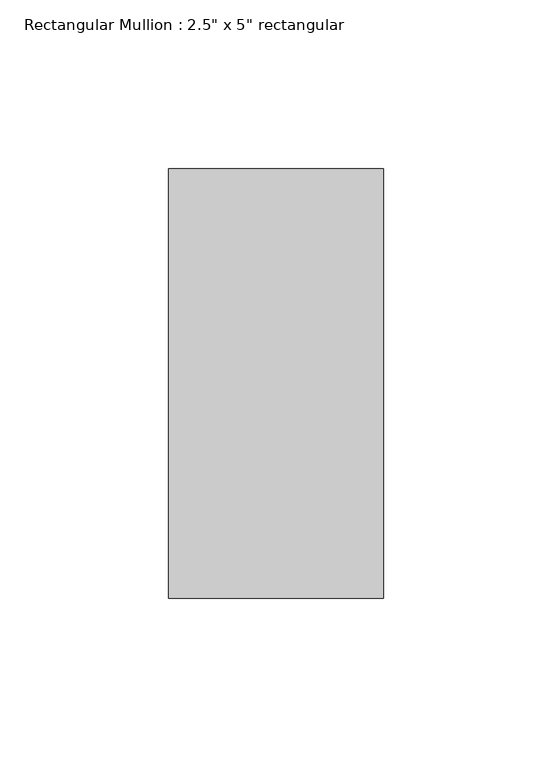
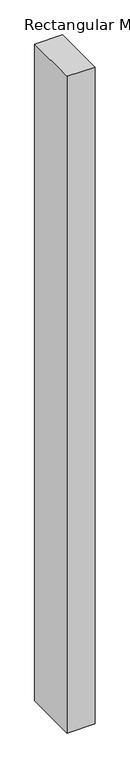
"""IFC4 building model written with IfcOpenShell, lengths in millimetres: member geometry."""

from ifc_helpers import new_model, si_unit, frame, origin, place, context, project, spatial, polyline, outline, extrude, source, transform, mapped, element, save


def member_1e2e73c0(model_context):
    return source(origin(), model_context, "Body", "SweptSolid", [
        extrude(outline(polyline([(31.75, 63.5), (31.75, -63.5), (-31.75, -63.5), (-31.75, 63.5), (31.75, 63.5)])), frame((0.0, 0.0, -1569.7635787), z_axis=(0.0, 0.0, 1.0), x_axis=(1.0, 0.0, 0.0)), (0.0, 0.0, 1.0), 1569.7635787),
    ])


if __name__ == "__main__":
    model = new_model("IFC4")
    model_context = context("Model", 3, world=origin())
    ifc_project = project(units=[si_unit("LENGTHUNIT", "METRE", prefix="MILLI")], contexts=[model_context])
    site = spatial("IfcSite", under=ifc_project)
    building = spatial("IfcBuilding", under=site)
    placement = place(None, origin())
    member_shape = member_1e2e73c0(model_context)
    element("IfcMember", 1, ObjectType="Rectangular Mullion : 2.5\" x 5\" rectangular", at=placement, inside=building, context=model_context, shape_type="MappedRepresentation", body=[
        mapped(member_shape, transform((0.0, 0.0, 0.0), x_axis=(1.0, 0.0, 0.0), y_axis=(0.0, 1.0, 0.0), z_axis=(0.0, 0.0, 1.0))),
    ])
    save(model, "model.ifc")

# Revit data of these elements
# Type "Rectangular Mullion : 2.5\" x 5\" rectangular"
#   built-in parameter 1007304 = 0.416667 (stored number, unit not read)
#   built-in parameter 1007301 = 0.104167 (stored number, unit not read)
#   built-in parameter 1007300 = 0.104167 (stored number, unit not read)
# Element 1 (IfcMember, "Rectangular Mullion : 2.5\" x 5\" rectangular")
#   Materials on its faces: "Aluminum"
# Materials
#   "Aluminum": class "Metal", colour RGB 247 247 247, transparency 0, Description = "Aluminum 6061", Cost = 0
